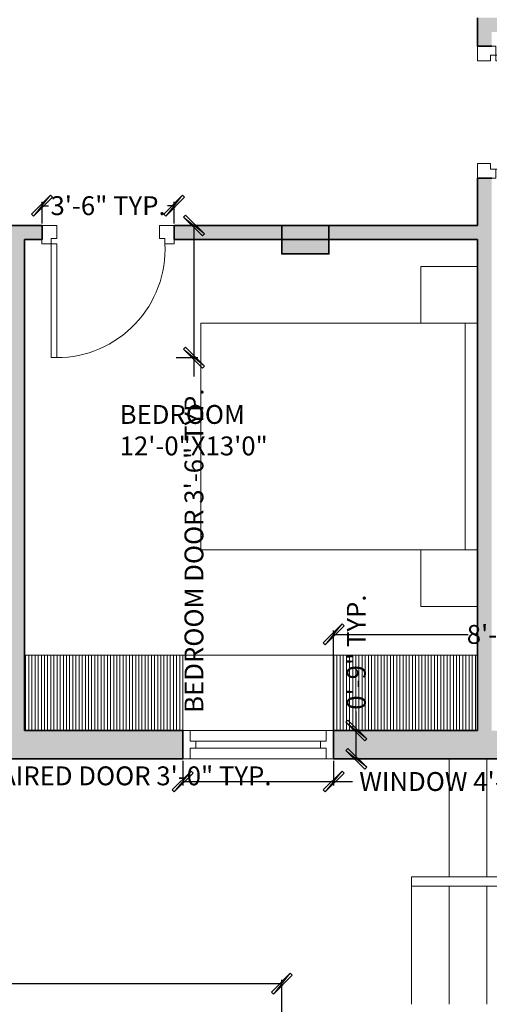
# Model space of a CAD drawing. Units: inches. Extents: x 1018 to 2596, y 723 to 1501.
# Tile 3 of 6: x 1276 to 1425, y 916 to 1229. Entities that reach past the tile are written whole.
import ezdxf

# ---------------------------------------------------------------- set-up
doc = ezdxf.new("R2010")
doc.units = ezdxf.units.IN
doc.layers.get('Defpoints').update_dxf_attribs({"lineweight": 0})
for name, color, linetype, lineweight in [('A-ANNO-DIMS', 2, 'Continuous', 13), ('A-AREA-IDEN', 7, 'Continuous', 18), ('A-COLS', 7, 'Continuous', 35), ('A-DOOR', 4, 'Continuous', 18), ('A-FLOR-CASE', 8, 'Continuous', 18), ('A-FLOR-CASE-PATT', 9, 'Continuous', 9), ('A-FLOR-STRS', 7, 'Continuous', 18), ('A-FURN', 8, 'Continuous', 13), ('A-WALL', 7, 'Continuous', 35), ('A-WINDOW', 4, 'Continuous', 13)]:
    doc.layers.add(name, color=color, linetype=linetype, lineweight=lineweight)
doc.layers.add('A-WALL-PATT', color=9, linetype='Continuous', lineweight=9, true_color=0xc7c8ca)
doc.styles.get("Standard").update_dxf_attribs({"font": 'arial.ttf'})
doc.dimstyles.new('saketh', dxfattribs={"dimtxt": 6, "dimasz": 6, "dimexe": 1.25, "dimexo": 0.625, "dimtad": 0, "dimdec": 1, "dimlunit": 4, "dimtxsty": 'Standard', "dimblk": 'ARCHTICK', "dimcen": 2.5, "dimclrd": 256, "dimclre": 1, "dimadec": 0, "dimazin": 0, "dimtfac": 1, "dimtdec": 1, "dimtmove": 0, "dimatfit": 3, "dimldrblk": 'ARCHTICK', "dimfxl": 1, "dimtolj": 1, "dimarcsym": 0})

# ---------------------------------------------------------------- blocks, each defined once
blk = doc.blocks.new('3 6 2')
at = {"layer": 'A-DOOR'}
for points in [[(-36.75, 5.83), (-36.75, 42), (-35, 42), (-35, 5.83)], [(-36.75, 4.08), (-35, 4.08), (-35, 0), (-39.67, 0), (-39.67, 5.83), (-36.75, 5.83)], [(-0.58, 5.83), (-0.58, 4.08), (-2.33, 4.08), (-2.33, 0), (2.33, 0), (2.33, 5.83)]]:
    blk.add_lwpolyline(points, close=True, dxfattribs=at)
at = {"layer": 'A-DOOR', "ltscale": 0.1}
blk.add_arc((-35, 7.54), 34.46, 357.1595, 90, dxfattribs=at)
blk = doc.blocks.new('BED')
at = {"layer": 'A-FURN'}
for points in [[(1841.83, 1404.74), (1769.83, 1404.74), (1769.83, 1488.74), (1841.83, 1488.74)], [(1769.83, 1400.81), (1751.83, 1400.81), (1751.83, 1418.81), (1769.83, 1418.81)], [(1841.83, 1400.81), (1859.83, 1400.81), (1859.83, 1418.81), (1841.83, 1418.81)], [(1769.83, 1404.74), (1841.83, 1404.74), (1841.83, 1400.81), (1769.83, 1400.81)]]:
    blk.add_lwpolyline(points, close=True, dxfattribs=at)
blk = doc.blocks.new('WINDOW FRAME')
at = {"layer": 'A-WINDOW'}
for points in [[(4180.39, 4970.76), (4180.39, 4972.59), (4178.2, 4972.59), (4178.2, 4970.76)], [(4178.2, 4970.76), (4174.8, 4970.76), (4174.8, 4968.41), (4183.8, 4968.41), (4183.8, 4970.76), (4180.39, 4970.76)]]:
    blk.add_lwpolyline(points, dxfattribs=at)
blk = doc.blocks.new("4' window")
at = {"layer": 'A-WINDOW'}
for p, q in [((2.35, 9), (45.65, 9)), ((43.82, 5.59), (4.18, 5.59)), ((43.82, 3.41), (4.18, 3.41)), ((2.35, 0), (45.65, 0))]:
    blk.add_line(p, q, dxfattribs=at)
at = {"layer": 'A-WINDOW', "rotation": 270}
blk.add_blockref('WINDOW FRAME', (-4968.41, 4183.8), dxfattribs=at)
at = {"layer": 'A-WINDOW', "xscale": -1, "rotation": 90}
blk.add_blockref('WINDOW FRAME', (5016.41, 4183.8), dxfattribs=at)
blk = doc.blocks.new('COLUMN-15X9-IN')
h = blk.add_hatch(color=256)
h.dxf.hatch_style = 1
h.paths.add_polyline_path([(15, 0), (15, 9), (0, 9), (0, 0)])
blk.add_lwpolyline([(15, 9), (15, 0), (0, 0), (0, 9)], close=True)
blk = doc.blocks.new('_ArchTick')
for p, q in [((0.447, 0.553), (-0.553, -0.447)), ((0.553, 0.447), (0.447, 0.553)), ((-0.447, -0.553), (0.553, 0.447)), ((-0.553, -0.447), (-0.447, -0.553))]:
    blk.add_line(p, q)
mesh = blk.add_polyface()
corners = [(-0.447, -0.553), (0.447, 0.553), (-0.553, -0.447), (0.553, 0.447)]
mesh.append_faces([[corners[k] for k in face] for face in [(0, 1, 2), (1, 0, 3)]], dxfattribs={"vtx0": -1})
blk = doc.blocks.new('*D59')
at = {"layer": 'A-ANNO-DIMS', "color": 1, "lineweight": -2, "transparency": 16777216}
for p, q in [((1219.19, 993.1), (1219.19, 987.08)), ((1255.19, 993.1), (1255.19, 987.08))]:
    blk.add_line(p, q, dxfattribs=at)
at = {"layer": 'A-ANNO-DIMS', "lineweight": -2, "transparency": 16777216}
for p, q in [((1219.19, 988.33), (1255.19, 988.33)), ((1255.19, 988.33), (1261.19, 988.33))]:
    blk.add_line(p, q, dxfattribs=at)
at = {"layer": 'Defpoints', "color": 0, "transparency": 16777216}
for p in [(1219.19, 993.73), (1255.19, 993.73), (1255.19, 988.33)]:
    blk.add_point(p, dxfattribs=at)
at = {"layer": 'A-ANNO-DIMS', "lineweight": -2, "transparency": 16777216, "xscale": 6, "yscale": 6, "zscale": 6, "rotation": 180}
blk.add_blockref('_ArchTick', (1219.19, 988.33), dxfattribs=at)
at = {"layer": 'A-ANNO-DIMS', "lineweight": -2, "transparency": 16777216, "xscale": 6, "yscale": 6, "zscale": 6}
blk.add_blockref('_ArchTick', (1255.19, 988.33), dxfattribs=at)
at = {"layer": 'A-ANNO-DIMS', "color": 0, "transparency": 16777216, "insert": (1310.45, 988.33), "char_height": 6, "attachment_point": 5}
blk.add_mtext('\\A1;PAIRED DOOR 3\'-0" TYP.', dxfattribs=at)
blk = doc.blocks.new('*D63')
at = {"layer": 'A-ANNO-DIMS', "color": 1, "lineweight": -2, "transparency": 16777216}
for p, q in [((1325.84, 1163.23), (1332.77, 1163.23)), ((1325.84, 1121.23), (1332.77, 1121.23))]:
    blk.add_line(p, q, dxfattribs=at)
at = {"layer": 'A-ANNO-DIMS', "lineweight": -2, "transparency": 16777216}
for p, q in [((1331.52, 1163.23), (1331.52, 1121.23)), ((1331.52, 1121.23), (1331.52, 1115.23))]:
    blk.add_line(p, q, dxfattribs=at)
at = {"layer": 'Defpoints', "color": 0, "transparency": 16777216}
for p in [(1325.22, 1163.23), (1325.22, 1121.23), (1331.52, 1121.23)]:
    blk.add_point(p, dxfattribs=at)
at = {"layer": 'A-ANNO-DIMS', "lineweight": -2, "transparency": 16777216, "xscale": 6, "yscale": 6, "zscale": 6}
for p, rotation in [((1331.52, 1163.23), 90), ((1331.52, 1121.23), 270)]:
    blk.add_blockref('_ArchTick', p, dxfattribs=dict(at, rotation=rotation))
at = {"layer": 'A-ANNO-DIMS', "color": 0, "transparency": 16777216, "insert": (1331.52, 1059.89), "char_height": 6, "attachment_point": 5, "rotation": 90}
blk.add_mtext('\\A1;BEDROOM DOOR 3\'-6" TYP.', dxfattribs=at)
blk = doc.blocks.new('*D64')
at = {"layer": 'A-ANNO-DIMS', "color": 1, "lineweight": -2, "transparency": 16777216}
for p, q in [((1283.22, 1163.85), (1283.22, 1170.78)), ((1325.22, 1163.85), (1325.22, 1170.78))]:
    blk.add_line(p, q, dxfattribs=at)
at = {"layer": 'A-ANNO-DIMS', "lineweight": -2, "transparency": 16777216}
for p, q in [((1283.22, 1169.53), (1285.31, 1169.53)), ((1325.22, 1169.53), (1323.13, 1169.53))]:
    blk.add_line(p, q, dxfattribs=at)
at = {"layer": 'Defpoints', "color": 0, "transparency": 16777216}
for p in [(1325.22, 1169.53), (1283.22, 1163.23), (1325.22, 1163.23)]:
    blk.add_point(p, dxfattribs=at)
at = {"layer": 'A-ANNO-DIMS', "lineweight": -2, "transparency": 16777216, "xscale": 6, "yscale": 6, "zscale": 6, "rotation": 180}
blk.add_blockref('_ArchTick', (1283.22, 1169.53), dxfattribs=at)
at = {"layer": 'A-ANNO-DIMS', "lineweight": -2, "transparency": 16777216, "xscale": 6, "yscale": 6, "zscale": 6}
blk.add_blockref('_ArchTick', (1325.22, 1169.53), dxfattribs=at)
at = {"layer": 'A-ANNO-DIMS', "color": 0, "transparency": 16777216, "insert": (1304.22, 1169.53), "char_height": 6, "attachment_point": 5}
blk.add_mtext('\\A1;3\'-6" TYP.', dxfattribs=at)
blk = doc.blocks.new('*D67')
at = {"layer": 'A-ANNO-DIMS', "color": 1, "lineweight": -2, "transparency": 16777216}
for p, q in [((1327.94, 993.1), (1327.94, 985.28)), ((1375.94, 993.1), (1375.94, 985.28))]:
    blk.add_line(p, q, dxfattribs=at)
at = {"layer": 'A-ANNO-DIMS', "lineweight": -2, "transparency": 16777216}
for p, q in [((1327.94, 986.53), (1375.94, 986.53)), ((1375.94, 986.53), (1381.94, 986.53))]:
    blk.add_line(p, q, dxfattribs=at)
at = {"layer": 'Defpoints', "color": 0, "transparency": 16777216}
for p in [(1327.94, 993.73), (1375.94, 993.73), (1375.94, 986.53)]:
    blk.add_point(p, dxfattribs=at)
at = {"layer": 'A-ANNO-DIMS', "lineweight": -2, "transparency": 16777216, "xscale": 6, "yscale": 6, "zscale": 6, "rotation": 180}
blk.add_blockref('_ArchTick', (1327.94, 986.53), dxfattribs=at)
at = {"layer": 'A-ANNO-DIMS', "lineweight": -2, "transparency": 16777216, "xscale": 6, "yscale": 6, "zscale": 6}
blk.add_blockref('_ArchTick', (1375.94, 986.53), dxfattribs=at)
at = {"layer": 'A-ANNO-DIMS', "color": 0, "transparency": 16777216, "insert": (1420.52, 986.53), "char_height": 6, "attachment_point": 5}
blk.add_mtext('\\A1;WINDOW 4\'-0" TYP.', dxfattribs=at)
blk = doc.blocks.new('*D68')
at = {"layer": 'A-ANNO-DIMS', "lineweight": -2, "transparency": 16777216}
for p, q in [((1383.14, 1002.73), (1383.14, 1008.73)), ((1383.14, 993.73), (1383.14, 1002.73))]:
    blk.add_line(p, q, dxfattribs=at)
at = {"layer": 'A-ANNO-DIMS', "color": 1, "lineweight": -2, "transparency": 16777216}
for p, q in [((1376.56, 1002.73), (1384.39, 1002.73)), ((1376.56, 993.73), (1384.39, 993.73))]:
    blk.add_line(p, q, dxfattribs=at)
at = {"layer": 'Defpoints', "color": 0, "transparency": 16777216}
for p in [(1375.94, 1002.73), (1383.14, 1002.73), (1375.94, 993.73)]:
    blk.add_point(p, dxfattribs=at)
at = {"layer": 'A-ANNO-DIMS', "lineweight": -2, "transparency": 16777216, "xscale": 6, "yscale": 6, "zscale": 6}
for p, rotation in [((1383.14, 1002.73), 90), ((1383.14, 993.73), 270)]:
    blk.add_blockref('_ArchTick', p, dxfattribs=dict(at, rotation=rotation))
at = {"layer": 'A-ANNO-DIMS', "color": 0, "transparency": 16777216, "insert": (1383.14, 1027.64), "char_height": 6, "attachment_point": 5, "rotation": 90}
blk.add_mtext('\\A1;0\'-9" TYP.', dxfattribs=at)
blk = doc.blocks.new('*D84')
at = {"layer": 'A-ANNO-DIMS', "color": 1, "lineweight": -2, "transparency": 16777216}
for p, q in [((1157.69, 883.35), (1157.69, 923.53)), ((1359.46, 883.35), (1359.46, 923.53))]:
    blk.add_line(p, q, dxfattribs=at)
at = {"layer": 'A-ANNO-DIMS', "lineweight": -2, "transparency": 16777216}
for p, q in [((1157.69, 922.28), (1245.6, 922.28)), ((1359.46, 922.28), (1271.55, 922.28))]:
    blk.add_line(p, q, dxfattribs=at)
at = {"layer": 'Defpoints', "color": 0, "transparency": 16777216}
for p in [(1359.46, 922.28), (1157.69, 882.73), (1359.46, 882.73)]:
    blk.add_point(p, dxfattribs=at)
at = {"layer": 'A-ANNO-DIMS', "lineweight": -2, "transparency": 16777216, "xscale": 6, "yscale": 6, "zscale": 6, "rotation": 180}
blk.add_blockref('_ArchTick', (1157.69, 922.28), dxfattribs=at)
at = {"layer": 'A-ANNO-DIMS', "lineweight": -2, "transparency": 16777216, "xscale": 6, "yscale": 6, "zscale": 6}
blk.add_blockref('_ArchTick', (1359.46, 922.28), dxfattribs=at)
at = {"layer": 'A-ANNO-DIMS', "color": 0, "transparency": 16777216, "insert": (1258.57, 922.28), "char_height": 6, "attachment_point": 5}
blk.add_mtext('\\A1;16\'-10"', dxfattribs=at)
blk = doc.blocks.new('*D89')
at = {"layer": 'A-ANNO-DIMS', "color": 1, "lineweight": -2, "transparency": 16777216}
for p, q in [((1375.94, 994.35), (1375.94, 1034.53)), ((1478.69, 994.35), (1478.69, 1034.53))]:
    blk.add_line(p, q, dxfattribs=at)
at = {"layer": 'A-ANNO-DIMS', "lineweight": -2, "transparency": 16777216}
for p, q in [((1375.94, 1033.28), (1418.71, 1033.28)), ((1478.69, 1033.28), (1435.92, 1033.28))]:
    blk.add_line(p, q, dxfattribs=at)
at = {"layer": 'Defpoints', "color": 0, "transparency": 16777216}
for p in [(1478.69, 1033.28), (1375.94, 993.73), (1478.69, 993.73)]:
    blk.add_point(p, dxfattribs=at)
at = {"layer": 'A-ANNO-DIMS', "lineweight": -2, "transparency": 16777216, "xscale": 6, "yscale": 6, "zscale": 6, "rotation": 180}
blk.add_blockref('_ArchTick', (1375.94, 1033.28), dxfattribs=at)
at = {"layer": 'A-ANNO-DIMS', "lineweight": -2, "transparency": 16777216, "xscale": 6, "yscale": 6, "zscale": 6}
blk.add_blockref('_ArchTick', (1478.69, 1033.28), dxfattribs=at)
at = {"layer": 'A-ANNO-DIMS', "color": 0, "transparency": 16777216, "insert": (1427.31, 1033.28), "char_height": 6, "attachment_point": 5}
blk.add_mtext('\\A1;8\'-7"', dxfattribs=at)

msp = doc.modelspace()

# ---------------------------------------------------------------- hatches: boundary and pattern name
at = {"layer": 'A-FLOR-CASE-PATT'}
h = msp.add_hatch(dxfattribs=at)
h.set_pattern_fill('_USER', color=256, angle=90, pattern_type=0)
h.set_pattern_definition([(90, (0, 0), (-1, 1e-16), [])])
h.paths.add_polyline_path([(1327.94, 1026.73), (1321.94, 1026.73), (1277.69, 1026.73), (1277.69, 1002.73), (1327.94, 1002.73)])
h.paths.add_polyline_path([(1421.69, 1026.73), (1381.94, 1026.73), (1375.94, 1026.73), (1375.94, 1002.73), (1421.69, 1002.73)])
at = {"layer": 'A-WALL-PATT', "transparency": 33554539}
h = msp.add_hatch(color=256, dxfattribs=at)
h.dxf.hatch_style = 1
h.paths.add_polyline_path([(1359.46, 1344.73), (1359.46, 1353.73), (1322.14, 1353.73), (1322.14, 1348.16), (1322.14, 1344.73)])
h.paths.add_polyline_path([(1374.46, 1353.73), (1374.46, 1344.73), (1421.69, 1344.73), (1421.69, 1296.73), (1415.69, 1296.73), (1415.69, 1292.23), (1426.19, 1292.23), (1426.19, 1344.73), (1568.69, 1344.73), (1568.69, 1353.73)])
h.paths.add_polyline_path([(1257.69, 1344.73), (1274.14, 1344.73), (1274.14, 1353.73), (1157.69, 1353.73), (1157.69, 1344.73)])
h.paths.add_polyline_path([(1151.69, 1344.73), (1142.69, 1344.73), (1142.69, 1257.11), (1148.25, 1257.11), (1151.69, 1257.11)])
h.paths.add_polyline_path([(1142.69, 1163.23), (1151.69, 1163.23), (1151.69, 1221.11), (1142.69, 1221.11)])
h.paths.add_polyline_path([(1151.69, 1154.23), (1142.69, 1154.23), (1142.69, 993.73), (1219.19, 993.73), (1219.19, 999.29), (1219.19, 1002.73), (1151.69, 1002.73)])
h.paths.add_polyline_path([(1327.94, 993.73), (1327.94, 1002.73), (1277.69, 1002.73), (1277.69, 1158.73), (1283.22, 1158.73), (1283.22, 1163.23), (1273.19, 1163.23), (1268.69, 1163.23), (1268.69, 1158.73), (1273.19, 1158.73), (1273.19, 1002.73), (1255.19, 1002.73), (1255.19, 993.73)])
h.paths.add_polyline_path([(1426.19, 1002.73), (1426.19, 1178.23), (1421.69, 1178.23), (1421.69, 1163.23), (1374.46, 1163.23), (1374.46, 1158.73), (1421.69, 1158.73), (1421.69, 1002.73), (1375.94, 1002.73), (1375.94, 993.73), (1478.69, 993.73), (1478.69, 1002.73)])
h.paths.add_polyline_path([(1583.69, 1233.73), (1574.69, 1233.73), (1574.69, 1229.23), (1421.69, 1229.23), (1421.69, 1220.23), (1426.19, 1220.23), (1426.19, 1224.73), (1480.19, 1224.73), (1480.19, 1158.73), (1489.19, 1158.73), (1489.19, 1163.23), (1484.69, 1163.23), (1484.69, 1224.73), (1508.69, 1224.73), (1574.69, 1224.73), (1574.69, 1163.23), (1583.69, 1163.23)])
h.paths.add_polyline_path([(1574.69, 1263.73), (1580.52, 1263.73), (1583.69, 1263.73), (1583.69, 1344.73), (1574.69, 1344.73)])
h.paths.add_polyline_path([(1583.69, 1154.23), (1574.69, 1154.23), (1574.69, 1002.73), (1583.69, 1002.73)])
h.paths.add_polyline_path([(1568.69, 993.73), (1568.69, 1002.73), (1526.69, 1002.73), (1526.69, 993.73)])
h.paths.add_polyline_path([(1359.46, 1158.73), (1359.46, 1163.23), (1325.22, 1163.23), (1325.22, 1158.73)])
h.paths.add_polyline_path([(1232.69, 1158.73), (1232.69, 1163.23), (1157.69, 1163.23), (1157.69, 1158.73)])

# ---------------------------------------------------------------- linework, layer by layer
at = {"layer": 'A-FLOR-CASE'}
for p, q in [((1321.94, 1026.73), (1277.69, 1026.73)), ((1321.94, 1026.73), (1381.94, 1026.73)), ((1327.94, 1026.73), (1327.94, 1002.73)), ((1375.94, 1026.73), (1375.94, 1002.73)), ((1421.69, 1026.73), (1381.94, 1026.73))]:
    msp.add_line(p, q, dxfattribs=at)
at = {"layer": 'A-FLOR-STRS'}
for p, q in [((1412.69, 993.73), (1412.69, 956.23)), ((1424.69, 993.73), (1424.69, 956.23)), ((1400.69, 956.23), (1400.69, 915.73)), ((1532.69, 956.23), (1400.69, 956.23)), ((1532.69, 953.23), (1400.69, 953.23)), ((1412.69, 953.23), (1412.69, 915.73)), ((1424.69, 953.23), (1424.69, 915.73))]:
    msp.add_line(p, q, dxfattribs=at)
at = {"layer": 'A-WALL'}
for p, q in [((1421.69, 1220.23), (1421.69, 1229.23)), ((1426.19, 1220.23), (1421.69, 1220.23)), ((1421.69, 1163.23), (1421.69, 1178.23)), ((1426.19, 1178.23), (1421.69, 1178.23)), ((1273.19, 1163.23), (1283.22, 1163.23)), ((1283.22, 1163.23), (1283.22, 1158.73)), ((1325.22, 1163.23), (1325.22, 1158.73)), ((1325.22, 1163.23), (1421.69, 1163.23)), ((1277.69, 1158.73), (1277.69, 1002.73)), ((1277.69, 1158.73), (1283.22, 1158.73)), ((1325.22, 1158.73), (1421.69, 1158.73)), ((1421.69, 1158.73), (1421.69, 1002.73)), ((1327.94, 1002.73), (1277.69, 1002.73)), ((1327.94, 1002.73), (1327.94, 993.73)), ((1421.69, 1002.73), (1375.94, 1002.73)), ((1375.94, 1002.73), (1375.94, 993.73)), ((1327.94, 993.73), (1255.19, 993.73)), ((1478.69, 993.73), (1375.94, 993.73))]:
    msp.add_line(p, q, dxfattribs=at)

# ---------------------------------------------------------------- block references
at = {"layer": 'A-COLS'}
msp.add_blockref('COLUMN-15X9-IN', (1359.46, 1154.22), dxfattribs=at)
at = {"layer": 'A-DOOR', "rotation": 270}
msp.add_blockref('3 6 2', (1421.69, 1180.56), dxfattribs=at)
at = {"layer": 'A-DOOR', "xscale": -1, "rotation": 180}
msp.add_blockref('3 6 2', (1322.88, 1163.23), dxfattribs=at)
at = {"layer": 'A-FURN', "rotation": 90}
msp.add_blockref('BED', (2822.5, -709.68), dxfattribs=at)
at = {"layer": 'A-WINDOW'}
msp.add_blockref("4' window", (1327.94, 993.73), dxfattribs=at)

# ---------------------------------------------------------------- texts
at = {"layer": 'A-AREA-IDEN', "insert": (1296.9, 1106.18), "char_height": 9, "attachment_point": 1}
msp.add_mtext_dynamic_manual_height_columns('\\A1;{\\H0.66667x;      BEDROOM\\P      12\'-0"X13\'0"}', width=129.8331, gutter_width=12.5, heights=[0], dxfattribs=at)

# ---------------------------------------------------------------- dimensions: what is measured, and where the dimension line sits
at = {"layer": 'A-ANNO-DIMS'}
for base, p1, p2, text, picture, middle in [((1325.22, 1169.53), (1283.22, 1163.23), (1325.22, 1163.23), '<> TYP.', '*D64', (1304.22, 1169.53)), ((1255.19, 988.33), (1219.19, 993.73), (1255.19, 993.73), 'PAIRED DOOR <> TYP.', '*D59', (1310.45, 988.33)), ((1375.94, 986.53), (1327.94, 993.73), (1375.94, 993.73), 'WINDOW <> TYP.', '*D67', (1420.52, 986.53))]:
    dim = msp.add_linear_dim(base=base, p1=p1, p2=p2, text=text, dimstyle='saketh', override={"dimdec": 1, "dimlfac": 1, "dimrnd": 0, "dimzin": 1, "dimdsep": 46, "dimlunit": 4, "dimfrac": 2}, dxfattribs=at)
    dim.commit()
    dim.dimension.update_dxf_attribs({"geometry": picture, "text_midpoint": middle})
for base, p1, p2, angle, text, picture, middle in [((1331.52, 1121.23), (1325.22, 1163.23), (1325.22, 1121.23), 270, 'BEDROOM DOOR <> TYP.', '*D63', (1331.52, 1059.89)), ((1383.14, 1002.73), (1375.94, 993.73), (1375.94, 1002.73), 90, '<> TYP.', '*D68', (1383.14, 1027.64))]:
    dim = msp.add_linear_dim(base=base, p1=p1, p2=p2, angle=angle, text=text, dimstyle='saketh', override={"dimdec": 1, "dimlfac": 1, "dimrnd": 0, "dimzin": 1, "dimdsep": 46, "dimlunit": 4, "dimfrac": 2}, dxfattribs=at)
    dim.commit()
    dim.dimension.update_dxf_attribs({"geometry": picture, "text_midpoint": middle})
dim = msp.add_linear_dim(base=(1478.686856, 1033.27536), p1=(1375.936856, 993.725361), p2=(1478.686856, 993.725359), angle=359.99999871, dimstyle='saketh', override={"dimdec": 1, "dimlfac": 1, "dimrnd": 0, "dimzin": 1, "dimdsep": 46, "dimlunit": 4, "dimfrac": 2}, dxfattribs=at)
dim.commit()
dim.dimension.update_dxf_attribs({"geometry": '*D89', "text_midpoint": (1427.311856, 1033.27536)})
dim = msp.add_linear_dim(base=(1359.46, 922.28), p1=(1157.69, 882.73), p2=(1359.46, 882.73), dimstyle='saketh', override={"dimdec": 1, "dimlfac": 1, "dimrnd": 0, "dimzin": 1, "dimdsep": 46, "dimlunit": 4, "dimfrac": 2}, dxfattribs=at)
dim.commit()
dim.dimension.update_dxf_attribs({"geometry": '*D84', "text_midpoint": (1258.57, 922.28)})

doc.saveas('drawing.dxf')
